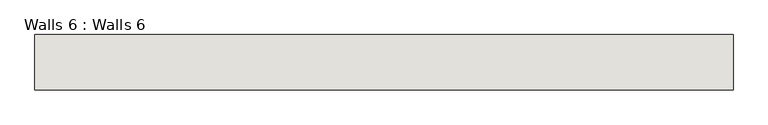
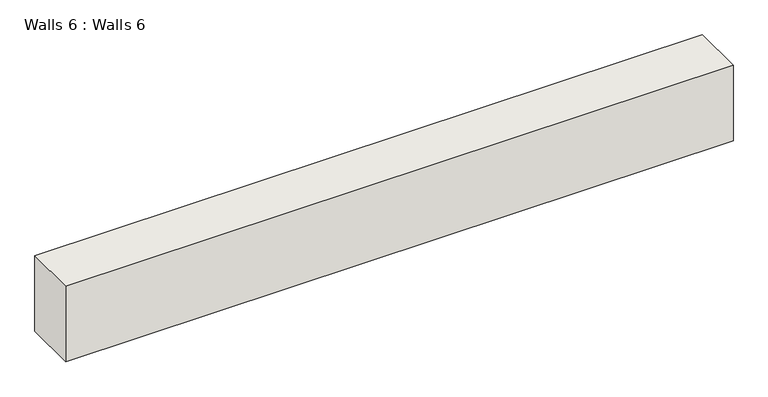
"""IFC4 building model written with IfcOpenShell, lengths in millimetres: wall geometry, Walls 6 : Walls 6."""

from ifc_helpers import new_model, si_unit, frame, origin, place, context, project, spatial, polyline, outline, extrude, source, transform, mapped, element, save


def walls_6_walls_6_35ebc142(model_context):
    return source(origin(), model_context, "Body", "SweptSolid", [
        extrude(outline(polyline([(-6719.1728698, -4040.6783675), (-8116.1728698, -4040.6783675), (-8116.1728698, -3929.6259649), (-6719.1728698, -3929.6259649), (-6719.1728698, -4040.6783675)])), frame((0.0, 0.0, 4840.3839838), z_axis=(0.0, 0.0, 1.0), x_axis=(1.0, 0.0, 0.0)), (0.0, 0.0, 1.0), 166.7365479),
    ])


if __name__ == "__main__":
    model = new_model("IFC4")
    model_context = context("Model", 3, world=origin())
    ifc_project = project(units=[si_unit("LENGTHUNIT", "METRE", prefix="MILLI")], contexts=[model_context])
    site = spatial("IfcSite", under=ifc_project)
    building = spatial("IfcBuilding", under=site)
    placement = place(None, origin())
    walls_6_walls_6_shape = walls_6_walls_6_35ebc142(model_context)
    element("IfcWall", 1, ObjectType="Walls 6 : Walls 6", at=placement, inside=building, context=model_context, shape_type="MappedRepresentation", body=[
        mapped(walls_6_walls_6_shape, transform((0.0, 0.0, 0.0), x_axis=(1.0, 0.0, 0.0), y_axis=(0.0, 1.0, 0.0), z_axis=(0.0, 0.0, 1.0))),
    ])
    save(model, "model.ifc")

# Revit data of these elements
# Element 1 (IfcWall, "Walls 6 : Walls 6")
#   Materials on its faces: "Default Wall"
# Materials
#   "Default Wall": colour RGB 128 128 128, transparency 0
